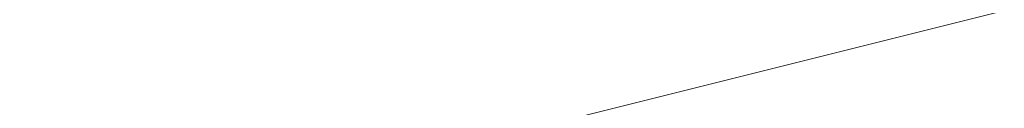
# Model space of a CAD drawing. Units: inches. Extents: x 2091 to 2899, y 967 to 2217.
# Tile 93 of 256: x 2251.2431 to 2251.3854, y 1099.9312 to 1099.9437. Entities that reach past the tile are written whole.
import ezdxf

# ---------------------------------------------------------------- set-up
doc = ezdxf.new("R2010")
doc.units = ezdxf.units.IN
doc.layers.add('A-ANNO-DIMS', color=2, linetype='Continuous', lineweight=18)
doc.layers.add('L-PLNT-TREE', color=94, linetype='Continuous', lineweight=13)
doc.layers.add('A-WALL-PATT', color=141, linetype='Continuous', lineweight=13, true_color=0xadddf7)
doc.styles.get("Standard").update_dxf_attribs({"font": 'arial.ttf'})
doc.dimstyles.new('ISO-25', dxfattribs={"dimtxt": 4, "dimasz": 4, "dimexe": 1.25, "dimexo": 0.625, "dimtad": 1, "dimdec": 0, "dimlunit": 3, "dimtxsty": 'Standard', "dimcen": 2.5, "dimadec": 0, "dimazin": 0, "dimtfac": 1, "dimtdec": 0, "dimtmove": 0, "dimatfit": 3, "dimfxl": 1, "dimarcsym": 0})

# ---------------------------------------------------------------- blocks, each defined once
blk = doc.blocks.new('*U29')
blk.add_line((-402.336, 12.192), (-451.104, 0))
blk = doc.blocks.new('*D71')
at = {"layer": 'A-ANNO-DIMS', "color": 0, "lineweight": -2, "transparency": 16777216}
for p, q in [((2212.1436, 1351.29406), (2212.1436, 969.4643)), ((2452.1436, 1351.29406), (2452.1436, 969.4643)), ((2216.1436, 970.7143), (2448.1436, 970.7143))]:
    blk.add_line(p, q, dxfattribs=at)
at = {"layer": 'A-ANNO-DIMS', "color": 0, "transparency": 16777216}
for points in [[(2216.1436, 971.38097), (2216.1436, 970.04764), (2212.1436, 970.7143)], [(2448.1436, 971.38097), (2448.1436, 970.04764), (2452.1436, 970.7143)]]:
    blk.add_solid(points, dxfattribs=at)
at = {"layer": 'Defpoints', "color": 0, "transparency": 16777216}
for p in [(2212.1436, 1351.91906), (2452.1436, 1351.91906), (2452.1436, 970.7143)]:
    blk.add_point(p, dxfattribs=at)
at = {"layer": 'A-ANNO-DIMS', "color": 0, "transparency": 16777216, "insert": (2332.1436, 973.38159), "char_height": 4, "attachment_point": 5}
blk.add_mtext('20\'-0"', dxfattribs=at)
blk = doc.blocks.new('*D75')
at = {"layer": 'A-ANNO-DIMS', "color": 0, "lineweight": -2, "transparency": 16777216}
for p, q in [((2212.1436, 1274.79406), (2212.1436, 969.4643)), ((2308.1436, 1274.79406), (2308.1436, 969.4643)), ((2216.1436, 970.7143), (2304.1436, 970.7143))]:
    blk.add_line(p, q, dxfattribs=at)
at = {"layer": 'A-ANNO-DIMS', "color": 0, "transparency": 16777216}
for points in [[(2216.1436, 971.38097), (2216.1436, 970.04764), (2212.1436, 970.7143)], [(2304.1436, 971.38097), (2304.1436, 970.04764), (2308.1436, 970.7143)]]:
    blk.add_solid(points, dxfattribs=at)
at = {"layer": 'Defpoints', "color": 0, "transparency": 16777216}
for p in [(2212.1436, 1275.41906), (2308.1436, 1275.41906), (2308.1436, 970.7143)]:
    blk.add_point(p, dxfattribs=at)
at = {"layer": 'A-ANNO-DIMS', "color": 0, "transparency": 16777216, "insert": (2260.1436, 973.38159), "char_height": 4, "attachment_point": 5}
blk.add_mtext('8\'-0"', dxfattribs=at)

msp = doc.modelspace()

# ---------------------------------------------------------------- hatches: boundary and pattern name
at = {"layer": 'A-WALL-PATT'}
h = msp.add_hatch(color=256, dxfattribs=at)
h.dxf.hatch_style = 1
h.paths.add_polyline_path([(2803.1436, 2050.91906), (2203.1436, 2050.91906), (2203.1436, 1090.91906), (2803.1436, 1090.91906)])
h.paths.add_polyline_path([(2635.79885, 1147.54046), (2674.52405, 1147.54046, 0.376086), (2678.52967, 1152.8802), (2678.52967, 1159.55647, 0.333335), (2674.52432, 1163.56185), (2674.52432, 1163.56185), (2674.52432, 1192.93439), (2635.80597, 1192.93439), (2597.08762, 1192.93439), (2597.08762, 1163.56185, 0.333335), (2593.08228, 1159.55647), (2593.08228, 1152.8802, 0.376086), (2597.08789, 1147.54046)], flags=0)
h.paths.add_polyline_path([(2436.01043, 1278.24078, 0.000483), (2435.95264, 1278.21503, -0.001328), (2435.93563, 1278.11169, -0.001711), (2436.11644, 1278.04076, 0.002185)], flags=0)
h.paths.add_polyline_path([(2794.1436, 1143.41906), (2794.1436, 1347.41906), (2543.37017, 1347.41906), (2543.37017, 1351.91906), (2794.1436, 1351.91906), (2794.1436, 1392.71355), (2793.9474, 1392.71355), (2793.9474, 1473.5369), (2794.1436, 1473.5369), (2794.1436, 1531.91906), (2650.1436, 1531.91906), (2650.1436, 1536.41906), (2794.1436, 1536.41906), (2794.1436, 1692.41906), (2609.37561, 1692.41906), (2609.37561, 1644.41906), (2604.87561, 1644.41906), (2604.87561, 1744.91906), (2609.37561, 1744.91906), (2609.37561, 1696.91906), (2794.1436, 1696.91906), (2794.1436, 1780.91906), (2609.6436, 1780.91906), (2493.87561, 1780.91906), (2493.87561, 1785.41906), (2609.6436, 1785.41906), (2794.1436, 1785.41906), (2794.1436, 1847.93882), (2793.95122, 1847.93882), (2793.95122, 1928.76217), (2794.1436, 1928.76217), (2794.1436, 1941.41906), (2614.1436, 1941.41906), (2614.1436, 1821.41906), (2609.6436, 1821.41906), (2609.6436, 1941.41906), (2392.1436, 1941.41906), (2392.1436, 1819.91906), (2387.6436, 1819.91906), (2387.6436, 1941.41906), (2212.1436, 1941.41906), (2212.1436, 1783.91906), (2392.1436, 1783.91906), (2392.1436, 1780.91906), (2212.1436, 1780.91906), (2212.1436, 1629.41906), (2387.6436, 1629.41906), (2387.6436, 1744.91906), (2392.1436, 1744.91906), (2392.1436, 1627.91906), (2317.1436, 1627.91906), (2317.1436, 1551.41906), (2317.1436, 1536.41906), (2459.38359, 1536.41906), (2459.38359, 1602.39648), (2463.88359, 1602.39648), (2463.88359, 1531.91906), (2456.6436, 1531.91906), (2456.6436, 1529.91906), (2452.1436, 1529.91906), (2452.1436, 1531.91906), (2312.6436, 1531.91906), (2312.6436, 1551.41906), (2306.1436, 1551.41906), (2306.1436, 1555.91906), (2308.1436, 1555.91906), (2308.1436, 1551.41906), (2312.6436, 1551.41906), (2312.6436, 1627.91906), (2212.1436, 1627.91906), (2212.1436, 1555.91906), (2270.1436, 1555.91906), (2270.1436, 1551.41906), (2212.1436, 1551.41906), (2212.1436, 1351.91906), (2272.1436, 1351.91906), (2272.1436, 1347.41906), (2212.1436, 1347.41906), (2212.1436, 1275.41906), (2308.1436, 1275.41906), (2308.1436, 1351.91906), (2452.1436, 1351.91906), (2452.1436, 1493.91906), (2456.6436, 1493.91906), (2456.6436, 1347.41906), (2312.6436, 1347.41906), (2312.6436, 1270.91906), (2212.1436, 1270.91906), (2212.1436, 1099.91906), (2281.23752, 1099.91906), (2282.87104, 1110.9138), (2282.00834, 1116.9966), (2278.55774, 1121.4204), (2268.20564, 1128.0562), (2272.08764, 1128.0562), (2273.81294, 1131.927), (2279.42034, 1134.6919), (2285.02784, 1135.2449), (2287.61584, 1137.4568), (2288.04714, 1138.0098), (2289.34114, 1140.7747), (2291.06654, 1139.6687), (2292.36054, 1135.2449), (2295.37984, 1136.9038), (2296.24254, 1135.7979), (2297.10524, 1133.033), (2300.12464, 1138.0098), (2303.14394, 1138.0098), (2304.43794, 1135.7979), (2303.14394, 1133.586), (2306.59464, 1134.6919), (2307.88874, 1133.033), (2310.90804, 1135.2449), (2313.92744, 1134.1389), (2315.62686, 1132.4271), (2308.32004, 1117.5496), (2290.20384, 1109.8079), (2288.90984, 1103.1721), (2289.27231, 1099.91906), (2434.91823, 1099.91906), (2431.59323, 1124.78806), (2429.93023, 1169.55306), (2430.92718, 1240.51969), (2435.65893, 1238.18613), (2437.13523, 1196.55406), (2438.79823, 1143.97306), (2442.67823, 1111.99806), (2446.55823, 1099.91906), (2794.1436, 1099.91906), (2794.1436, 1138.91906), (2548.03245, 1138.91906), (2548.03245, 1143.41906), (2548.03245, 1148.81906), (2546.66846, 1148.03156), (2528.68569, 1179.17862, 0.256256), (2512.03245, 1148.81906), (2512.03245, 1143.41906), (2512.03245, 1138.91906), (2507.53245, 1138.91906), (2507.53245, 1143.41906), (2507.53245, 1148.81906, 0.256256), (2490.8792, 1179.17862), (2472.89644, 1148.03156), (2471.53245, 1148.81906), (2471.53245, 1143.41906), (2467.03245, 1143.41906), (2467.03245, 1269.94579, 0.039061), (2460.90999, 1273.58006), (2467.03245, 1273.58006), (2467.03245, 1286.32536, 0.014511), (2465.21619, 1286.76191), (2467.03245, 1287.05258), (2467.03245, 1323.41906), (2471.53245, 1323.41906), (2471.53245, 1148.81906), (2489.53245, 1179.99597), (2490.89644, 1179.20847), (2490.8792, 1179.17862, -0.256256), (2507.53245, 1148.81906), (2507.53245, 1143.41906), (2512.03245, 1143.41906), (2512.03245, 1148.81906, -0.256256), (2528.68569, 1179.17862), (2528.66846, 1179.20847), (2530.03245, 1179.99597), (2548.03245, 1148.81906), (2548.03245, 1143.41906)], flags=16)
h.paths.add_polyline_path([(2607.76855, 1200.94508), (2607.76855, 1265.03063), (2597.08762, 1281.05201), (2619.78459, 1281.05201), (2627.79528, 1337.12686), (2635.79885, 1337.12686), (2643.81666, 1337.12686), (2651.82736, 1281.05201), (2674.52432, 1281.05201), (2663.8434, 1265.03063), (2663.8434, 1200.94508), (2635.80597, 1200.94508)], flags=0)
edge = h.paths.add_edge_path(flags=0)
edge.add_ellipse((13303.89622, 1272.99872), major_axis=(-10595.31304, 0), ratio=0.84230387009, start_angle=0.628237219, end_angle=0.6465541, ccw=False)
edge.add_ellipse((2711.70045, 1156.85268), major_axis=(2.21977, 0), ratio=0.8423039, start_angle=111.53524, end_angle=180.62824, ccw=False)
edge.add_ellipse((13303.15629, 1272.99872), major_axis=(-10593.02631, 0), ratio=0.84230386954, start_angle=0.528271472, end_angle=0.646554097, ccw=False)
edge.add_line((2710.7646, 1175.3333), (2710.12999, 1175.3333))
edge.add_ellipse((2710.12999, 1176.57978), major_axis=(1.47985, 0), ratio=0.8423039, start_angle=180, end_angle=270, ccw=False)
edge.add_line((2708.65014, 1176.57978), (2708.65014, 1200.78291))
edge.add_ellipse((2710.12999, 1200.78291), major_axis=(1.47985, 0), ratio=0.8423039, start_angle=90, end_angle=180, ccw=False)
edge.add_line((2710.12999, 1202.02939), (2710.46508, 1202.02939))
edge.add_ellipse((13303.15629, 1272.99872), major_axis=(-10593.02631, 0), ratio=0.84230386954, start_angle=-0.090229089, end_angle=0.383866779, ccw=False)
edge.add_ellipse((2710.12999, 1290.92703), major_axis=(-1.47985, 0), ratio=0.8423039, start_angle=0, end_angle=90, ccw=False)
edge.add_line((2708.65014, 1290.92703), (2708.65014, 1315.13017))
edge.add_ellipse((2710.12999, 1315.13017), major_axis=(-1.47985, 0), ratio=0.8423039, start_angle=-90, end_angle=0, ccw=False)
edge.add_line((2710.12999, 1316.37665), (2710.70631, 1316.37665))
edge.add_ellipse((3238.40172, 1296.28957), major_axis=(528.234, 0), ratio=0.84230387, start_angle=176.3495724, end_angle=177.8200497, ccw=False)
edge.add_ellipse((2775.06304, 1071.4507), major_axis=(313.30776, 0), ratio=0.84230387, start_angle=102.1259656, end_angle=103.780529, ccw=False)
edge.add_ellipse((2775.06304, 1078.3057), major_axis=(-305.30289, 0), ratio=0.84230387, start_angle=-79.790461, end_angle=-77.5553727, ccw=False)
edge.add_ellipse((2695.14177, 1541.97538), major_axis=(-250.96022, 0), ratio=0.84230387, start_angle=99.256566, end_angle=102.5549326)
edge.add_line((2741.41033, 1334.21426), (2747.13255, 1337.37848))
edge.add_ellipse((2747.53862, 1336.85748), major_axis=(-0.73992, 0), ratio=0.842304, start_angle=270, end_angle=307.93313, ccw=False)
edge.add_ellipse((2747.53862, 1336.85748), major_axis=(-0.73992, 0), ratio=0.842304, start_angle=232.06687, end_angle=270, ccw=False)
edge.add_line((2747.94469, 1337.37848), (2753.66691, 1334.21426))
edge.add_ellipse((2799.93547, 1541.97538), major_axis=(250.96022, 0), ratio=0.84230387, start_angle=257.4450674, end_angle=260.743434)
edge.add_ellipse((2720.01419, 1078.3057), major_axis=(305.30289, 0), ratio=0.84230387, start_angle=77.5553727, end_angle=79.790461, ccw=False)
edge.add_ellipse((2720.01419, 1071.4507), major_axis=(-313.30776, 0), ratio=0.84230387, start_angle=256.219471, end_angle=257.8740344, ccw=False)
edge.add_ellipse((2256.67551, 1296.28957), major_axis=(-528.234, 0), ratio=0.84230387, start_angle=182.1799503, end_angle=183.6504276, ccw=False)
edge.add_line((2784.37092, 1316.37665), (2784.94725, 1316.37665))
edge.add_ellipse((2784.94725, 1315.13017), major_axis=(1.47985, 0), ratio=0.8423039, start_angle=0, end_angle=90, ccw=False)
edge.add_line((2786.42709, 1315.13017), (2786.42709, 1290.92703))
edge.add_ellipse((2784.94725, 1290.92703), major_axis=(1.47985, 0), ratio=0.8423039, start_angle=270, end_angle=360, ccw=False)
edge.add_ellipse((-7808.07906, 1272.99872), major_axis=(10593.02631, 0), ratio=0.84230386954, start_angle=-0.383866779, end_angle=0.090229089, ccw=False)
edge.add_line((2784.61216, 1202.02939), (2784.94725, 1202.02939))
edge.add_ellipse((2784.94725, 1200.78291), major_axis=(1.47985, 0), ratio=0.8423039, start_angle=0, end_angle=90, ccw=False)
edge.add_line((2786.42709, 1200.78291), (2786.42709, 1176.57978))
edge.add_ellipse((2784.94725, 1176.57978), major_axis=(-1.47985, 0), ratio=0.8423039, start_angle=90, end_angle=180, ccw=False)
edge.add_line((2784.94725, 1175.3333), (2784.31264, 1175.3333))
edge.add_ellipse((-7808.07906, 1272.99872), major_axis=(10593.02631, 0), ratio=0.84230386954, start_angle=-0.618643196, end_angle=-0.528271472, ccw=False)
edge.add_ellipse((2783.37678, 1156.85268), major_axis=(-2.21977, 0), ratio=0.8423039, start_angle=179.37176, end_angle=248.46476, ccw=False)
edge.add_ellipse((-7808.81898, 1272.99872), major_axis=(-10595.31304, 0), ratio=0.84230386576, start_angle=179.353445923, end_angle=179.371762803, ccw=False)
edge.add_ellipse((2780.2973, 1153.50079), major_axis=(-5.24643, 0), ratio=0.8423039, start_angle=90, end_angle=179.35345, ccw=False)
edge.add_line((2780.2973, 1149.08171), (2714.77993, 1149.08171))
edge.add_ellipse((2714.77993, 1153.50079), major_axis=(5.24643, 0), ratio=0.8423039, start_angle=180.64655, end_angle=270, ccw=False)
edge = h.paths.add_edge_path(flags=0)
edge.add_line((2718.18737, 1151.00783), (2718.18737, 1170.47236))
edge.add_ellipse((2721.14706, 1170.47236), major_axis=(-2.95969, 0), ratio=0.8423039, start_angle=-90, end_angle=0, ccw=False)
edge.add_line((2721.14706, 1172.96532), (2773.93017, 1172.96532))
edge.add_ellipse((2773.93017, 1170.47236), major_axis=(-2.95969, 0), ratio=0.8423039, start_angle=180, end_angle=270, ccw=False)
edge.add_line((2776.88987, 1170.47236), (2776.88987, 1151.00783))
edge.add_line((2776.88987, 1151.00783), (2718.18737, 1151.00783))
edge = h.paths.add_edge_path(flags=0)
edge.add_line((2718.18737, 1180.23415), (2718.18737, 1199.05783))
edge.add_ellipse((2747.53862, 1320.39864), major_axis=(147.01792, 0), ratio=0.84230387, start_angle=256.4018653, end_angle=283.5981347)
edge.add_line((2776.88987, 1199.05783), (2776.88987, 1180.23415))
edge.add_ellipse((2747.53862, 1301.57496), major_axis=(147.01792, 0), ratio=0.84230387, start_angle=256.4018653, end_angle=283.5981347, ccw=False)
edge = h.paths.add_edge_path(flags=0)
edge.add_ellipse((13303.15629, 1272.99872), major_axis=(-10591.54646, 0), ratio=0.84230386955, start_angle=0.055594314, end_angle=0.377764194, ccw=False)
edge.add_line((2711.61686, 1262.72171), (2715.66741, 1249.4954))
edge.add_ellipse((6413.89196, 1241.69192), major_axis=(-3698.23616, 0), ratio=0.8423038695, start_angle=-0.12089737, end_angle=0.36407635)
edge.add_line((2715.76104, 1218.19245), (2711.93431, 1203.16736))
edge = h.paths.add_edge_path(flags=0)
edge.add_line((2718.18737, 1251.07457), (2716.00249, 1267.45044))
edge.add_ellipse((2742.15117, 1202.18954), major_axis=(81.77258, 0), ratio=0.84230387, start_angle=94.277421, end_angle=111.8349538, ccw=False)
edge.add_line((2737.00975, 1270.93063), (2758.06748, 1270.93063))
edge.add_ellipse((2752.92606, 1202.18954), major_axis=(81.77258, 0), ratio=0.84230387, start_angle=68.1650462, end_angle=85.722579, ccw=False)
edge.add_line((2779.07475, 1267.45044), (2776.88987, 1251.07457))
edge.add_ellipse((2750.33806, 1187.88536), major_axis=(79.57966, 0), ratio=0.84230387, start_angle=67.2080851, end_angle=85.1299304)
edge.add_line((2756.03466, 1254.74366), (2739.04258, 1254.74366))
edge.add_ellipse((2744.73917, 1187.88536), major_axis=(79.57966, 0), ratio=0.84230387, start_angle=94.8700696, end_angle=112.7919149)
edge = h.paths.add_edge_path(flags=0)
edge.add_line((2783.14293, 1203.16736), (2779.31619, 1218.19245))
edge.add_ellipse((-918.81473, 1241.69192), major_axis=(3698.23616, 0), ratio=0.8423038695, start_angle=-0.36407635, end_angle=0.12089737)
edge.add_line((2779.40983, 1249.4954), (2783.46037, 1262.72171))
edge.add_ellipse((-7808.07906, 1272.99872), major_axis=(-10591.54646, 0), ratio=0.84230386954, start_angle=179.622235806, end_angle=179.944405687, ccw=False)
edge = h.paths.add_edge_path(flags=0)
edge.add_ellipse((2734.20089, 1286.69044), major_axis=(-0.35661, 6.34008), ratio=0.6038336, start_angle=89.002014, end_angle=253.657408, ccw=False)
edge.add_line((2730.369, 1286.54181), (2730.369, 1301.35198))
edge.add_line((2730.369, 1301.35198), (2735.91331, 1305.2148))
edge.add_ellipse((2736.38492, 1304.73456), major_axis=(0.73992, 0), ratio=0.842304, start_angle=90, end_angle=134.48021, ccw=False)
edge.add_line((2736.38492, 1305.3578), (2738.03278, 1305.3578))
edge.add_line((2738.03278, 1305.3578), (2738.03278, 1307.70793))
edge.add_ellipse((2794.20164, 1307.70793), major_axis=(56.16886, 0), ratio=0.84230387, start_angle=150.56143, end_angle=180, ccw=False)
edge.add_ellipse((2700.87559, 1307.70793), major_axis=(-56.16886, 0), ratio=0.84230387, start_angle=180, end_angle=209.43857, ccw=False)
edge.add_line((2757.04445, 1307.70793), (2757.04445, 1305.3578))
edge.add_line((2757.04445, 1305.3578), (2758.69232, 1305.3578))
edge.add_ellipse((2758.69232, 1304.73456), major_axis=(-0.73992, 0), ratio=0.842304, start_angle=225.51979, end_angle=270, ccw=False)
edge.add_line((2759.16392, 1305.2148), (2764.70823, 1301.35198))
edge.add_line((2764.70823, 1301.35198), (2764.70823, 1286.54181))
edge.add_ellipse((2760.87634, 1286.69044), major_axis=(0.35661, 6.34008), ratio=0.6038336, start_angle=106.342592, end_angle=270.997986, ccw=False)
edge.add_line((2757.04445, 1285.79709), (2757.04445, 1307.70793))
edge.add_ellipse((2700.87559, 1307.70793), major_axis=(-56.16886, 0), ratio=0.84230387, start_angle=180, end_angle=209.43857)
edge.add_ellipse((2794.20164, 1307.70793), major_axis=(56.16886, 0), ratio=0.84230387, start_angle=150.56143, end_angle=180)
edge.add_line((2738.03278, 1307.70793), (2738.03278, 1285.79709))
h.paths.add_polyline_path([(2417.81227, 1104.4497), (2413.49227, 1102.5297), (2410.61227, 1103.9697), (2409.17227, 1106.3697), (2407.25227, 1107.3297), (2406.29227, 1109.7297), (2405.33227, 1114.0497), (2405.33227, 1117.8897), (2406.29227, 1120.1297), (2407.25227, 1119.8097), (2408.84832, 1118.32766), (2410.17395, 1119.42417), (2410.21127, 1120.4057), (2411.04073, 1121.41905), (2410.69927, 1119.8587), (2410.17395, 1119.42417), (2410.08845, 1117.17611), (2411.13284, 1116.20632), (2413.97227, 1119.3297), (2416.85227, 1120.7697), (2416.86972, 1120.79878), (2417.03507, 1119.40512), (2417.89621, 1118.14338), (2418.29227, 1118.3697), (2419.54445, 1120.03927), (2419.36092, 1118.38749), (2419.03211, 1119.35615), (2418.39894, 1118.51193), (2419.25227, 1114.5297), (2418.79409, 1107.19879)], flags=0)
h.paths.add_polyline_path([(2508.87017, 1347.41906), (2508.37017, 1347.41906), (2508.37017, 1351.91906), (2508.87017, 1351.91906)], flags=0)
h.paths.add_polyline_path([(2473.37017, 1347.41906), (2472.37017, 1347.41906), (2467.87017, 1347.41906), (2467.87017, 1455.41906), (2472.37017, 1455.41906), (2472.37017, 1352.41906), (2473.37017, 1352.41906)], flags=0)
h.paths.add_polyline_path([(2352.10624, 1217.4462), (2349.22624, 1218.8862), (2347.78624, 1221.2862), (2345.86624, 1222.2462), (2344.90624, 1224.6462), (2343.94624, 1228.9662), (2343.94624, 1232.8062), (2344.90624, 1235.0462), (2345.86624, 1234.7262), (2347.46229, 1233.24415), (2348.78792, 1234.34066), (2348.82524, 1235.3222), (2349.6547, 1236.33555), (2349.31324, 1234.7752), (2348.78792, 1234.34066), (2348.70242, 1232.0926), (2349.74681, 1231.12282), (2352.58624, 1234.2462), (2355.46624, 1235.6862), (2355.48369, 1235.71528), (2355.64904, 1234.32161), (2356.51018, 1233.05988), (2356.90624, 1233.2862), (2358.15842, 1234.95576), (2357.97489, 1233.30398), (2357.64608, 1234.27264), (2357.01291, 1233.42842), (2357.86624, 1229.4462), (2357.40806, 1222.11529), (2356.42624, 1219.3662)], flags=0)
h.paths.add_polyline_path([(2348.2968, 1112.22442), (2347.0138, 1112.31042), (2345.5298, 1114.12742), (2345.7318, 1115.85842), (2346.8118, 1116.98242), (2346.8118, 1114.64642), (2345.8668, 1114.21442), (2346.8798, 1114.30042)], flags=0)
h.paths.add_polyline_path([(2347.0138, 1110.92642), (2346.2718, 1110.49342), (2346.6098, 1111.18642)], flags=0)
h.paths.add_polyline_path([(2345.8668, 1118.19442), (2345.5298, 1117.32942), (2343.7078, 1118.02142), (2344.3828, 1118.62642)], flags=0)
h.paths.add_polyline_path([(2346.6768, 1109.28242), (2346.0698, 1108.07142), (2345.8668, 1110.06142)], flags=0)
h.paths.add_polyline_path([(2345.0568, 1119.75142), (2343.6398, 1119.75142), (2343.9778, 1121.13542)], flags=0)
h.paths.add_polyline_path([(2345.2598, 1116.55042), (2345.1248, 1115.85842), (2344.9218, 1115.68542), (2344.7198, 1116.37742)], flags=0)
h.paths.add_polyline_path([(2345.6648, 1112.31042), (2345.4618, 1111.53242), (2344.0448, 1111.96442), (2344.6518, 1112.57042)], flags=0)
h.paths.add_polyline_path([(2345.1918, 1113.34942), (2344.4498, 1113.86842), (2344.7198, 1114.38742)], flags=0)
h.paths.add_polyline_path([(2344.6518, 1116.80942), (2344.1798, 1115.68542), (2344.6518, 1115.33942), (2343.9098, 1114.90642), (2343.0328, 1115.94442), (2343.6398, 1116.46342)], flags=0)
h.paths.add_polyline_path([(2345.8668, 1106.68642), (2344.9898, 1105.56242), (2344.5168, 1106.60042)], flags=0)
h.paths.add_polyline_path([(2344.8548, 1110.06142), (2344.5168, 1109.28242), (2344.1128, 1109.71542)], flags=0)
h.paths.add_polyline_path([(2344.0448, 1113.52242), (2343.4378, 1113.08942), (2342.7628, 1113.95442)], flags=0)
h.paths.add_polyline_path([(2344.3148, 1111.01242), (2342.9648, 1110.32042), (2342.9648, 1111.09942)], flags=0)
h.paths.add_polyline_path([(2345.1248, 1104.69742), (2344.5848, 1103.74542), (2344.4498, 1104.26442)], flags=0)
h.paths.add_polyline_path([(2342.8298, 1121.22242), (2341.7498, 1120.53042), (2340.5358, 1121.04942), (2340.1308, 1121.82842), (2340.6708, 1122.95242), (2341.1428, 1121.82842), (2341.6148, 1122.00142)], flags=0)
h.paths.add_polyline_path([(2342.9648, 1119.75142), (2343.0328, 1118.45342), (2342.0878, 1118.02142), (2342.0198, 1119.49142)], flags=0)
h.paths.add_polyline_path([(2342.6948, 1116.89642), (2341.9528, 1116.63642), (2342.0198, 1117.32942)], flags=0)
h.paths.add_polyline_path([(2343.0328, 1112.22442), (2342.0198, 1111.79142), (2341.5478, 1112.22442), (2342.3578, 1113.34942)], flags=0)
h.paths.add_polyline_path([(2343.7748, 1104.43742), (2342.6278, 1102.88042), (2342.6948, 1104.61042), (2343.4378, 1105.12942)], flags=0)
h.paths.add_polyline_path([(2342.0198, 1115.07942), (2340.8058, 1115.51242), (2340.9408, 1116.37742)], flags=0)
h.paths.add_polyline_path([(2341.4808, 1120.09742), (2341.4808, 1119.40542), (2341.0758, 1119.57842), (2341.1428, 1120.09742)], flags=0)
h.paths.add_polyline_path([(2341.8178, 1114.47342), (2340.9408, 1113.08942), (2340.8058, 1114.56042)], flags=0)
h.paths.add_polyline_path([(2341.1428, 1118.54042), (2340.9408, 1116.98242), (2339.0508, 1117.67542), (2339.0508, 1118.62642)], flags=0)
h.paths.add_polyline_path([(2342.6948, 1101.66842), (2341.9528, 1101.84142), (2342.5598, 1102.36142)], flags=0)
h.paths.add_polyline_path([(2340.3328, 1119.66542), (2338.4438, 1119.57842), (2337.9038, 1120.35742), (2339.6578, 1120.61642)], flags=0)
h.paths.add_polyline_path([(2340.3328, 1115.33942), (2340.0628, 1113.69542), (2339.3878, 1115.33942)], flags=0)
h.paths.add_polyline_path([(2341.8178, 1103.83142), (2341.5478, 1102.88042), (2341.1428, 1103.65842)], flags=0)
h.paths.add_polyline_path([(2339.0508, 1122.86642), (2337.2958, 1121.82842), (2337.0938, 1123.12542), (2337.7688, 1123.81842)], flags=0)
h.paths.add_polyline_path([(2339.1178, 1121.74142), (2338.8478, 1121.22242), (2338.1738, 1121.04942), (2338.3758, 1121.56842)], flags=0)
h.paths.add_polyline_path([(2339.1858, 1119.31942), (2338.6458, 1118.71342), (2338.2408, 1118.10742), (2338.2408, 1118.88642)], flags=0)
h.paths.add_polyline_path([(2341.1428, 1101.92842), (2340.6028, 1101.23642), (2340.0628, 1101.84142), (2340.6028, 1102.36142)], flags=0)
h.paths.add_polyline_path([(2337.6338, 1117.76142), (2336.6208, 1118.28042), (2337.2958, 1118.97242)], flags=0)
h.paths.add_polyline_path([(2336.8238, 1119.57842), (2334.7988, 1118.97242), (2335.2038, 1120.35742), (2336.5538, 1120.87642)], flags=0)
h.paths.add_polyline_path([(2339.1178, 1100.45742), (2337.3638, 1100.54342), (2336.7558, 1101.23642)], flags=0)
h.paths.add_polyline_path([(2336.3508, 1122.43342), (2336.0138, 1121.91442), (2334.9338, 1122.43342), (2334.5288, 1123.47142), (2335.7438, 1122.77942)], flags=0)
h.paths.add_polyline_path([(2334.7318, 1120.87642), (2334.2588, 1120.35742), (2334.0568, 1120.78942), (2334.5968, 1121.30842)], flags=0)
h.paths.add_polyline_path([(2334.4618, 1122.17442), (2332.5718, 1121.30842), (2331.3568, 1122.17442), (2332.0998, 1122.86642)], flags=0)
h.paths.add_polyline_path([(2334.2588, 1118.54042), (2333.3818, 1118.45342), (2333.6518, 1119.31942)], flags=0)
h.paths.add_polyline_path([(2335.5418, 1102.27442), (2334.1918, 1102.62042), (2335.2718, 1103.31242)], flags=0)
h.paths.add_polyline_path([(2332.7068, 1119.66542), (2331.6948, 1120.44342), (2332.5048, 1120.78942)], flags=0)
h.paths.add_polyline_path([(2334.7318, 1101.14942), (2333.5168, 1101.58242), (2333.9888, 1101.75542)], flags=0)
h.paths.add_polyline_path([(2332.6398, 1116.63642), (2331.0868, 1116.29042), (2331.9648, 1118.19442)], flags=0)
h.paths.add_polyline_path([(2330.7498, 1121.56842), (2330.2768, 1120.27042), (2328.5228, 1119.31942), (2328.9948, 1121.04942)], flags=0)
h.paths.add_polyline_path([(2330.7498, 1118.62642), (2330.0078, 1117.50242), (2329.8728, 1118.02142)], flags=0)
h.paths.add_polyline_path([(2332.0998, 1102.36142), (2330.5468, 1102.01442), (2331.6948, 1102.96642)], flags=0)
h.paths.add_polyline_path([(2329.5348, 1113.60842), (2329.0628, 1112.31042), (2328.5898, 1113.34942)], flags=0)
h.paths.add_polyline_path([(2328.3878, 1117.84842), (2327.5098, 1116.55042), (2327.1728, 1117.76142)], flags=0)
h.paths.add_polyline_path([(2329.7378, 1106.51342), (2329.5348, 1105.30242), (2328.2528, 1106.08142)], flags=0)
h.paths.add_polyline_path([(2328.6578, 1114.38742), (2328.0498, 1114.12742), (2328.3198, 1114.90642)], flags=0)
h.paths.add_polyline_path([(2328.3198, 1112.22442), (2327.1058, 1112.13742), (2326.7008, 1112.65642)], flags=0)
h.paths.add_polyline_path([(2326.9028, 1115.25242), (2326.7008, 1114.12742), (2325.2158, 1113.60842), (2326.0928, 1115.33942)], flags=0)
h.paths.add_polyline_path([(2326.6328, 1108.33042), (2326.0928, 1107.37942), (2325.8908, 1108.50342), (2326.4978, 1109.10942)], flags=0)
h.paths.add_polyline_path([(2615.1436, 1531.91906), (2609.6436, 1531.91906), (2609.6436, 1620.41906), (2614.1436, 1620.41906), (2614.1436, 1536.41906), (2615.1436, 1536.41906)], flags=0)
h.paths.add_polyline_path([(2545.1436, 1563.41906), (2464.1436, 1563.41906), (2464.1436, 1632.41906), (2509.1436, 1632.41906), (2509.1436, 1627.91906), (2509.1436, 1603.91906), (2468.6436, 1603.91906), (2468.6436, 1567.91906), (2540.6436, 1567.91906), (2540.6436, 1591.91906), (2545.1436, 1591.91906)], flags=0)
h.paths.add_polyline_path([(2388.96905, 1549.98573), (2357.43418, 1549.98573), (2357.43418, 1623.36078), (2399.36278, 1623.36078), (2435.68947, 1623.36078), (2435.59255, 1602.55927), (2435.59255, 1602.39648), (2388.96905, 1602.39648)], flags=0)
h.paths.add_polyline_path([(2388.88063, 1555.80915), (2374.90443, 1555.80915), (2374.90443, 1600.57156), (2374.90443, 1615.45765), (2406.35088, 1615.45765), (2406.35088, 1618.93943), (2412.17429, 1615.45765), (2406.35088, 1611.97586), (2406.35088, 1615.45765), (2388.88063, 1615.45765)], flags=0)
h.paths.add_polyline_path([(2568.87561, 1644.41906), (2453.37561, 1644.41906), (2453.37561, 1785.41906), (2457.87561, 1785.41906), (2457.87561, 1648.91906), (2568.87561, 1648.91906)], flags=0)
h.paths.add_polyline_path([(2212.1436, 1945.91906), (2212.1436, 2041.91906), (2794.1436, 2041.91906), (2794.1436, 1945.91906)], flags=16)
h.paths.add_polyline_path([(2271.08273, 1964.31724), (2776.85297, 1964.31724), (2776.85297, 2037.16962), (2271.08273, 2037.16962)], flags=8)
h.paths.add_polyline_path([(2380.64929, 1536.82414), (2461.04081, 1536.82414), (2461.04081, 1554.65259), (2380.64929, 1554.65259)], flags=8)
h.paths.add_polyline_path([(2240.75571, 1609.72545), (2309.18583, 1609.72545), (2309.18583, 1617.6982), (2240.75571, 1617.6982)], flags=8)
h.paths.add_polyline_path([(2212.67726, 1313.5041), (2282.59152, 1313.5041), (2282.59152, 1322.74524), (2212.67726, 1322.74524)], flags=8)
h.paths.add_polyline_path([(2457.11198, 1114.77857), (2558.48158, 1114.77857), (2558.48158, 1142.21968), (2457.11198, 1142.21968)], flags=8)
h.paths.add_polyline_path([(2473.44234, 1273.01007), (2604.64123, 1273.01007), (2604.64123, 1318.34693), (2473.44234, 1318.34693)], flags=8)
h.paths.add_polyline_path([(2638.8763, 1626.97743), (2684.25037, 1627.97674), (2684.03848, 1637.59749), (2638.66442, 1636.59819)], flags=8)
h.paths.add_polyline_path([(2537.59055, 1453.79345), (2628.38955, 1453.79345), (2628.38955, 1475.34481), (2537.59055, 1475.34481)], flags=8)
h.paths.add_polyline_path([(2504.13764, 1714.6324), (2554.64719, 1714.6324), (2554.64719, 1730.23771), (2504.13764, 1730.23771)], flags=8)
h.paths.add_polyline_path([(2487.50118, 1575.65187), (2535.09712, 1575.65187), (2535.09712, 1598.37765), (2487.50118, 1598.37765)], flags=8)
h.paths.add_polyline_path([(2709.0994, 1735.71028), (2740.0166, 1735.71028), (2740.0166, 1749.93764), (2709.0994, 1749.93764)], flags=8)
h.paths.add_polyline_path([(2442.43842, 1792.17166), (2564.72884, 1792.17166), (2564.72884, 1842.00016), (2442.43842, 1842.00016)], flags=8)
h.paths.add_polyline_path([(2655.8158, 1809.64408), (2789.52014, 1806.6938), (2790.08498, 1832.29164), (2656.38064, 1835.24192)], flags=8)
h.paths.add_polyline_path([(2234.8427, 1797.72014), (2368.59285, 1794.76885), (2369.16072, 1820.50413), (2235.41056, 1823.45542)], flags=8)
h.paths.add_polyline_path([(2245.13847, 1644.00633), (2398.42773, 1640.6239), (2398.99484, 1666.32482), (2245.70557, 1669.70725)], flags=8)
h.paths.add_polyline_path([(2306.14285, 1431.16852), (2413.76831, 1428.79369), (2414.33315, 1454.39153), (2306.70768, 1456.76636)], flags=8)
h.paths.add_polyline_path([(2306.83458, 1458.23314), (2393.38048, 1456.32345), (2393.93281, 1481.35436), (2307.38691, 1483.26405)], flags=8)

# ---------------------------------------------------------------- block references
at = {"layer": 'L-PLNT-TREE', "xscale": 0.0393700787401575, "yscale": 0.0393700787401575, "zscale": 0.0393700787401575}
msp.add_blockref('*U29', (2269.04101, 1099.91906), dxfattribs=at)

# ---------------------------------------------------------------- dimensions: what is measured, and where the dimension line sits
at = {"layer": 'A-ANNO-DIMS'}
for base, p1, p2, picture, middle in [((2452.1436, 970.7143), (2212.1436, 1351.91906), (2452.1436, 1351.91906), '*D71', (2332.1436, 973.38159)), ((2308.1436, 970.7143), (2212.1436, 1275.41906), (2308.1436, 1275.41906), '*D75', (2260.1436, 973.38159))]:
    dim = msp.add_linear_dim(base=base, p1=p1, p2=p2, dimstyle='ISO-25', override={"dimdec": 1, "dimlfac": 1, "dimrnd": 0, "dimzin": 1, "dimdsep": 46, "dimlunit": 4, "dimfrac": 2}, dxfattribs=at)
    dim.commit()
    dim.dimension.update_dxf_attribs({"geometry": picture, "text_midpoint": middle})

doc.saveas('drawing.dxf')
